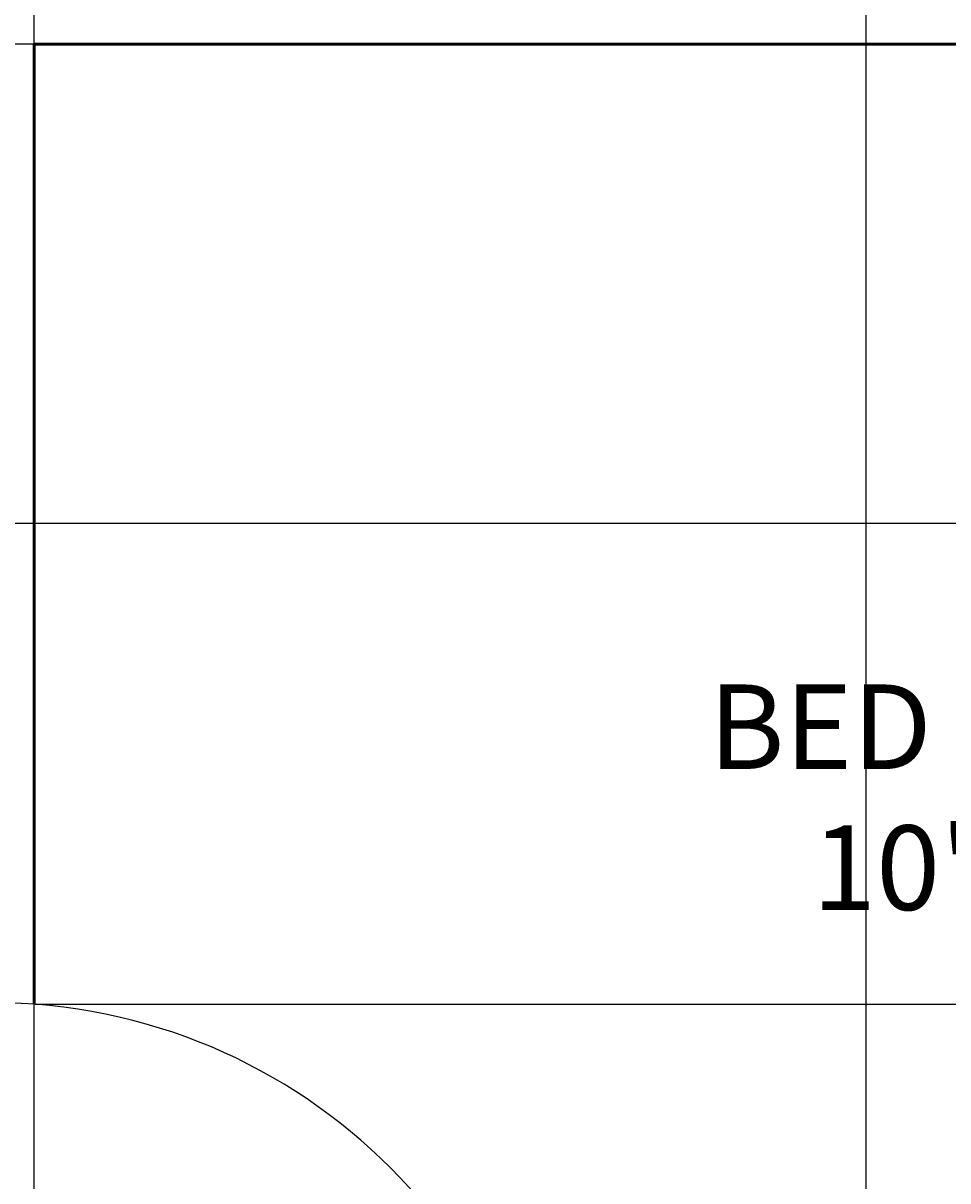
# Model space of a CAD drawing. Units: inches. Extents: x 37 to 824, y -700 to 234.
# Tile 62 of 77: x 298 to 364, y -75 to 8. Entities that reach past the tile are written whole.
import ezdxf

# ---------------------------------------------------------------- set-up
doc = ezdxf.new("R2010")
doc.units = ezdxf.units.IN
doc.header["$MEASUREMENT"] = 0
for name, color, linetype, lineweight in [('A-ANNO-DIMS', 2, 'Continuous', 18), ('A-AREA-IDEN', 3, 'Continuous', 18), ('A-DOOR', 4, 'Continuous', 25), ('A-WALL', 2, 'Continuous', 50)]:
    doc.layers.add(name, color=color, linetype=linetype, lineweight=lineweight)
doc.styles.get("Standard").update_dxf_attribs({"font": 'arial.ttf'})
doc.dimstyles.get("Standard").update_dxf_attribs({"dimtxt": 0.18, "dimasz": 0.18, "dimexe": 0.18, "dimexo": 0.0625, "dimgap": 0.09, "dimtad": 0, "dimtih": 1, "dimtoh": 1, "dimdec": 1, "dimzin": 0, "dimdsep": 46, "dimlunit": 4, "dimtxsty": 'Standard', "dimcen": 0.09, "dimadec": 0, "dimazin": 0, "dimtfac": 1, "dimtdec": 1, "dimtofl": 0, "dimtmove": 0, "dimatfit": 3, "dimfxl": 1, "dimtolj": 1, "dimtzin": 0, "dimarcsym": 0})

# ---------------------------------------------------------------- blocks, each defined once
blk = doc.blocks.new('*U5')
for p, q in [((0, 0), (0, 6)), ((40, 0), (40, 6))]:
    blk.add_line(p, q)
blk.add_lwpolyline([(0, 0), (0, -40), (1.75, -40), (1.75, 0)], close=True)
blk.add_arc((0, 0), 40, 270, 0)
blk = doc.blocks.new('*D62')
at = {"layer": 'A-ANNO-DIMS', "color": 0, "lineweight": -2, "ltscale": 0.5, "transparency": 16777216}
for p, q in [((419.015, 6.09), (78.159, 6.09)), ((78.339, 5.91), (78.339, -10.728)), ((78.339, -27.73), (78.339, -11.091)), ((419.015, -27.91), (78.159, -27.91))]:
    blk.add_line(p, q, dxfattribs=at)
at = {"layer": 'A-ANNO-DIMS', "color": 0, "ltscale": 0.5, "transparency": 16777216}
for points in [[(78.309, 5.91), (78.369, 5.91), (78.339, 6.09)], [(78.309, -27.73), (78.369, -27.73), (78.339, -27.91)]]:
    blk.add_solid(points, dxfattribs=at)
at = {"layer": 'Defpoints', "color": 0, "ltscale": 0.5, "transparency": 16777216}
for p in [(419.077, 6.09), (78.339, -27.91), (419.077, -27.91)]:
    blk.add_point(p, dxfattribs=at)
at = {"layer": 'A-ANNO-DIMS', "color": 0, "ltscale": 0.5, "transparency": 16777216, "insert": (78.339, -10.91), "char_height": 0.18, "attachment_point": 5}
blk.add_mtext('\\A1;2\'-10"', dxfattribs=at)
blk = doc.blocks.new('*D79')
at = {"layer": 'A-ANNO-DIMS', "color": 0, "lineweight": -2, "ltscale": 0.5, "transparency": 16777216}
for p, q in [((299.14, -62.022), (513.773, -62.022)), ((513.593, -62.202), (513.593, -81.784)), ((513.593, -101.73), (513.593, -82.148)), ((296.14, -101.91), (513.773, -101.91))]:
    blk.add_line(p, q, dxfattribs=at)
at = {"layer": 'A-ANNO-DIMS', "color": 0, "ltscale": 0.5, "transparency": 16777216}
for points in [[(513.563, -62.202), (513.623, -62.202), (513.593, -62.022)], [(513.563, -101.73), (513.623, -101.73), (513.593, -101.91)]]:
    blk.add_solid(points, dxfattribs=at)
at = {"layer": 'Defpoints', "color": 0, "ltscale": 0.5, "transparency": 16777216}
for p in [(299.077, -62.022), (296.077, -101.91), (513.593, -101.91)]:
    blk.add_point(p, dxfattribs=at)
at = {"layer": 'A-ANNO-DIMS', "color": 0, "ltscale": 0.5, "transparency": 16777216, "insert": (513.593, -81.966), "char_height": 0.18, "attachment_point": 5}
blk.add_mtext('\\A1;3\'-4"', dxfattribs=at)
blk = doc.blocks.new('*D82')
at = {"layer": 'A-ANNO-DIMS', "color": 0, "lineweight": -2, "ltscale": 0.5, "transparency": 16777216}
for p, q in [((299.077, -206.847), (299.077, 234.17)), ((358.132, -206.847), (358.132, 234.17)), ((299.257, 233.99), (328.202, 233.99)), ((357.952, 233.99), (329.008, 233.99))]:
    blk.add_line(p, q, dxfattribs=at)
at = {"layer": 'A-ANNO-DIMS', "color": 0, "ltscale": 0.5, "transparency": 16777216}
for points in [[(299.257, 234.02), (299.257, 233.96), (299.077, 233.99)], [(357.952, 234.02), (357.952, 233.96), (358.132, 233.99)]]:
    blk.add_solid(points, dxfattribs=at)
at = {"layer": 'Defpoints', "color": 0, "ltscale": 0.5, "transparency": 16777216}
for p in [(358.132, 233.99), (299.077, -206.91), (358.132, -206.91)]:
    blk.add_point(p, dxfattribs=at)
at = {"layer": 'A-ANNO-DIMS', "color": 0, "ltscale": 0.5, "transparency": 16777216, "insert": (328.605, 233.99), "char_height": 0.18, "attachment_point": 5}
blk.add_mtext('\\A1;4\'-11"', dxfattribs=at)
blk = doc.blocks.new('*D83')
at = {"layer": 'A-ANNO-DIMS', "color": 0, "lineweight": -2, "ltscale": 0.5, "transparency": 16777216}
for p, q in [((358.132, -206.847), (358.132, 234.17)), ((419.077, -206.847), (419.077, 234.17)), ((358.312, 233.99), (388.275, 233.99)), ((418.897, 233.99), (388.934, 233.99))]:
    blk.add_line(p, q, dxfattribs=at)
at = {"layer": 'A-ANNO-DIMS', "color": 0, "ltscale": 0.5, "transparency": 16777216}
for points in [[(358.312, 234.02), (358.312, 233.96), (358.132, 233.99)], [(418.897, 234.02), (418.897, 233.96), (419.077, 233.99)]]:
    blk.add_solid(points, dxfattribs=at)
at = {"layer": 'Defpoints', "color": 0, "ltscale": 0.5, "transparency": 16777216}
for p in [(419.077, 233.99), (358.132, -206.91), (419.077, -206.91)]:
    blk.add_point(p, dxfattribs=at)
at = {"layer": 'A-ANNO-DIMS', "color": 0, "ltscale": 0.5, "transparency": 16777216, "insert": (388.605, 233.99), "char_height": 0.18, "attachment_point": 5}
blk.add_mtext('\\A1;5\'-1"', dxfattribs=at)

msp = doc.modelspace()

# ---------------------------------------------------------------- linework, layer by layer
at = {"layer": 'A-WALL'}
for p in [(419.077, 6.09), (299.077, -62.022)]:
    msp.add_line(p, (299.077, 6.09), dxfattribs=at)

# ---------------------------------------------------------------- block references
at = {"layer": 'A-DOOR', "rotation": 90}
msp.add_blockref('*U5', (296.077, -101.91), dxfattribs=at)

# ---------------------------------------------------------------- texts
at = {"layer": 'A-AREA-IDEN', "insert": (346.954, -39.332), "char_height": 6, "attachment_point": 1}
msp.add_mtext_dynamic_manual_height_columns("BED ROOM\\P    10' X 9'", width=88.32168, gutter_width=1, heights=[0], dxfattribs=at)

# ---------------------------------------------------------------- dimensions: what is measured, and where the dimension line sits
at = {"layer": 'A-ANNO-DIMS', "ltscale": 0.5}
for base, p1, p2, picture, middle in [((358.132, 233.99), (299.077, -206.91), (358.132, -206.91), '*D82', (328.605, 233.99)), ((419.077, 233.99), (358.132, -206.91), (419.077, -206.91), '*D83', (388.605, 233.99))]:
    dim = msp.add_linear_dim(base=base, p1=p1, p2=p2, dimstyle='Standard', override={"dimdec": 1, "dimlfac": 1, "dimrnd": 0, "dimzin": 1, "dimdsep": 46, "dimlunit": 4, "dimfrac": 2}, dxfattribs=at)
    dim.commit()
    dim.dimension.update_dxf_attribs({"geometry": picture, "text_midpoint": middle})
for base, p1, p2, picture, middle in [((78.339, -27.91), (419.077, 6.09), (419.077, -27.91), '*D62', (78.339, -10.91)), ((513.593, -101.91), (299.077, -62.022), (296.077, -101.91), '*D79', (513.593, -81.966))]:
    dim = msp.add_linear_dim(base=base, p1=p1, p2=p2, angle=90, dimstyle='Standard', override={"dimdec": 1, "dimlfac": 1, "dimrnd": 0, "dimzin": 1, "dimdsep": 46, "dimlunit": 4, "dimfrac": 2}, dxfattribs=at)
    dim.commit()
    dim.dimension.update_dxf_attribs({"geometry": picture, "text_midpoint": middle})

doc.saveas('drawing.dxf')
